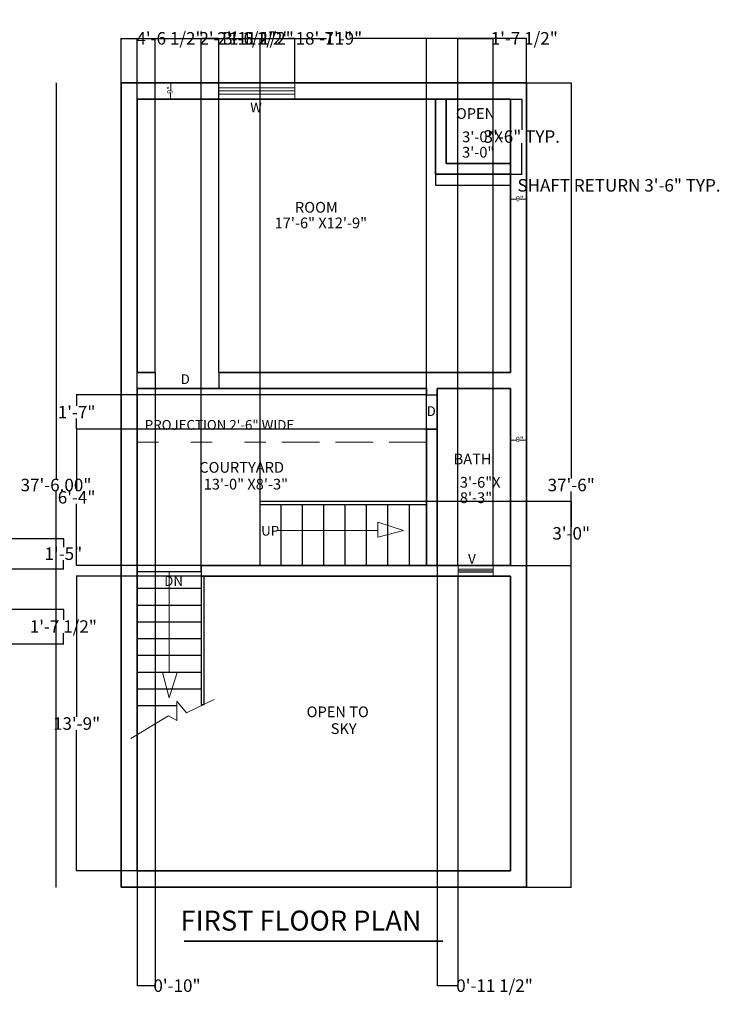
# Model space of a CAD drawing. Units: inches. Extents: x 193743 to 194406, y 400309 to 400860.
# Tile 2 of 2: x 194014 to 194406, y 400309 to 400860. Entities that reach past the tile are written whole.
import ezdxf

# ---------------------------------------------------------------- set-up
doc = ezdxf.new("R2010")
doc.units = ezdxf.units.IN
doc.header["$MEASUREMENT"] = 0
doc.linetypes.add('ACAD_ISO03W100', pattern=[30, 12, -18])
for name, color, linetype, lineweight in [('A-ANNO-DIMS', 2, 'Continuous', 18), ('A-ANNO-SYMB', 7, 'Continuous', 18), ('A-ANNO-TEXT', 7, 'Continuous', 18), ('A-ANNO-TITL', 7, 'Continuous', 35), ('A-AREA-IDEN', 7, 'Continuous', 18), ('A-DOOR', 3, 'Continuous', 25), ('A-FLOR-OVHD', 8, 'ACAD_ISO03W100', 18), ('A-FLOR-STRS', 7, 'Continuous', 25), ('A-GLAZ', 4, 'Continuous', 18), ('A-WALL', 7, 'Continuous', 35)]:
    doc.layers.add(name, color=color, linetype=linetype, lineweight=lineweight)
doc.styles.get("Standard").update_dxf_attribs({"font": 'arial.ttf'})
doc.dimstyles.get("Standard").update_dxf_attribs({"dimtxt": 7, "dimasz": 0.18, "dimexe": 0.18, "dimexo": 0.0625, "dimgap": 0.09, "dimtad": 0, "dimtih": 1, "dimtoh": 1, "dimzin": 0, "dimdsep": 46, "dimlunit": 3, "dimtxsty": 'Standard', "dimcen": 0.09, "dimadec": 0, "dimazin": 0, "dimtfac": 1, "dimtofl": 0, "dimtmove": 0, "dimatfit": 3, "dimfxl": 1, "dimtolj": 1, "dimtzin": 0, "dimarcsym": 0})

# ---------------------------------------------------------------- blocks, each defined once
blk = doc.blocks.new('*D2')
at = {"layer": 'A-ANNO-DIMS', "color": 0, "lineweight": -2, "transparency": 16777216}
for p, q in [((194034.37, 400824.24), (194034.71, 400824.24)), ((194034.53, 400824.06), (194034.53, 400602.91)), ((194034.53, 400374.42), (194034.53, 400595.57)), ((194034.37, 400374.24), (194034.71, 400374.24))]:
    blk.add_line(p, q, dxfattribs=at)
at = {"layer": 'A-ANNO-DIMS', "color": 0, "lineweight": 100, "transparency": 16777216}
for points in [[(194034.5, 400824.06), (194034.56, 400824.06), (194034.53, 400824.24)], [(194034.5, 400374.42), (194034.56, 400374.42), (194034.53, 400374.24)]]:
    blk.add_solid(points, dxfattribs=at)
at = {"layer": 'Defpoints', "color": 0, "lineweight": 100, "transparency": 16777216}
for p in [(194034.3, 400824.24), (194034.3, 400374.24), (194034.53, 400374.24)]:
    blk.add_point(p, dxfattribs=at)
at = {"layer": 'A-ANNO-DIMS', "color": 0, "transparency": 16777216, "insert": (194034.53, 400599.24), "char_height": 7, "attachment_point": 5}
blk.add_mtext('\\A1;37\'-6.00"', dxfattribs=at)
blk = doc.blocks.new('SHAFT-RETURN-36X36')
for p, q in [((0, 42), (0, 0)), ((6, 42), (6, 6)), ((6, 6), (42, 6)), ((0, 0), (42, 0))]:
    blk.add_line(p, q)
blk = doc.blocks.new('STAIR-DIRECTION-ARROW')
for p, q in [((3.8, 70.54), (3.8, 14.31)), ((0, 14.31), (8.31, 14.31)), ((3.8, 0), (0, 14.31)), ((8.31, 14.31), (3.8, 0))]:
    blk.add_line(p, q)
blk = doc.blocks.new('THICKNESS-9-H')
for p, q in [((0, 1.15), (3.54, 1.15)), ((5.14, 1.15), (9, 1.15))]:
    blk.add_line(p, q)
blk.add_text('9"', height=3).set_placement((2.97, 0))
blk = doc.blocks.new('THICKNESS-9-V')
for p, q in [((0.06, 9), (0.06, 5.01)), ((0, 3.6), (0, 0))]:
    blk.add_line(p, q)
blk.add_text('9"', height=3, rotation=90).set_placement((1.05, 2.9))
blk = doc.blocks.new('ROOM-TAG-OPEN-3X3')
for s, p in [('OPEN', (0, 21.67)), ('3\'-0"X', (3.49, 8.63)), ('3\'-0"', (3.46, 0))]:
    blk.add_text(s, height=6).set_placement(p)
blk = doc.blocks.new('*D10')
at = {"layer": 'A-ANNO-DIMS', "color": 0, "lineweight": -2, "transparency": 16777216}
for p, q in [((194247, 400773.18), (194247, 400766.76)), ((194289, 400773.18), (194289, 400766.76)), ((194247.18, 400766.94), (194288.82, 400766.94)), ((194289, 400766.94), (194289.18, 400766.94))]:
    blk.add_line(p, q, dxfattribs=at)
at = {"layer": 'A-ANNO-DIMS', "color": 0, "lineweight": 100, "transparency": 16777216}
for points in [[(194247.18, 400766.97), (194247.18, 400766.91), (194247, 400766.94)], [(194288.82, 400766.97), (194288.82, 400766.91), (194289, 400766.94)]]:
    blk.add_solid(points, dxfattribs=at)
at = {"layer": 'Defpoints', "color": 0, "lineweight": 100, "transparency": 16777216}
for p in [(194247, 400773.24), (194289, 400773.24), (194289, 400766.94)]:
    blk.add_point(p, dxfattribs=at)
at = {"layer": 'A-ANNO-DIMS', "color": 0, "transparency": 16777216, "insert": (194349.71, 400766.94), "char_height": 7, "attachment_point": 5}
blk.add_mtext('\\A1;SHAFT RETURN 3\'-6" TYP.', dxfattribs=at)
blk = doc.blocks.new('*D11')
at = {"layer": 'A-ANNO-DIMS', "color": 0, "lineweight": -2, "transparency": 16777216}
for p, q in [((194289.06, 400815.24), (194295.48, 400815.24)), ((194295.3, 400815.06), (194295.3, 400797.91)), ((194295.3, 400773.42), (194295.3, 400790.57)), ((194289.06, 400773.24), (194295.48, 400773.24))]:
    blk.add_line(p, q, dxfattribs=at)
at = {"layer": 'A-ANNO-DIMS', "color": 0, "lineweight": 100, "transparency": 16777216}
for points in [[(194295.27, 400815.06), (194295.33, 400815.06), (194295.3, 400815.24)], [(194295.27, 400773.42), (194295.33, 400773.42), (194295.3, 400773.24)]]:
    blk.add_solid(points, dxfattribs=at)
at = {"layer": 'Defpoints', "color": 0, "lineweight": 100, "transparency": 16777216}
for p in [(194289, 400815.24), (194295.3, 400815.24), (194289, 400773.24)]:
    blk.add_point(p, dxfattribs=at)
at = {"layer": 'A-ANNO-DIMS', "color": 0, "transparency": 16777216, "insert": (194295.3, 400794.24), "char_height": 7, "attachment_point": 5}
blk.add_mtext('\\A1;3\'-6" TYP.', dxfattribs=at)
blk = doc.blocks.new('*D14')
at = {"layer": 'A-ANNO-DIMS', "color": 0, "lineweight": -2, "transparency": 16777216}
for p, q in [((194071, 400824.3), (194071, 400849.37)), ((194071.18, 400849.19), (194170, 400849.19)), ((194297.82, 400849.19), (194199, 400849.19)), ((194298, 400824.3), (194298, 400849.37))]:
    blk.add_line(p, q, dxfattribs=at)
at = {"layer": 'A-ANNO-DIMS', "color": 0, "lineweight": 100, "transparency": 16777216}
for points in [[(194071.18, 400849.22), (194071.18, 400849.16), (194071, 400849.19)], [(194297.82, 400849.22), (194297.82, 400849.16), (194298, 400849.19)]]:
    blk.add_solid(points, dxfattribs=at)
at = {"layer": 'Defpoints', "color": 0, "lineweight": 100, "transparency": 16777216}
for p in [(194298, 400849.19), (194071, 400824.24), (194298, 400824.24)]:
    blk.add_point(p, dxfattribs=at)
at = {"layer": 'A-ANNO-DIMS', "color": 0, "transparency": 16777216, "insert": (194184.5, 400849.19), "char_height": 7, "attachment_point": 5}
blk.add_mtext('\\A1;18\'-11"', dxfattribs=at)
blk = doc.blocks.new('*D15')
at = {"layer": 'A-ANNO-DIMS', "color": 0, "lineweight": -2, "transparency": 16777216}
for p, q in [((194298.06, 400824.24), (194323.13, 400824.24)), ((194322.95, 400824.06), (194322.95, 400602.91)), ((194322.95, 400374.42), (194322.95, 400595.57)), ((194298.06, 400374.24), (194323.13, 400374.24))]:
    blk.add_line(p, q, dxfattribs=at)
at = {"layer": 'A-ANNO-DIMS', "color": 0, "lineweight": 100, "transparency": 16777216}
for points in [[(194322.92, 400824.06), (194322.98, 400824.06), (194322.95, 400824.24)], [(194322.92, 400374.42), (194322.98, 400374.42), (194322.95, 400374.24)]]:
    blk.add_solid(points, dxfattribs=at)
at = {"layer": 'Defpoints', "color": 0, "lineweight": 100, "transparency": 16777216}
for p in [(194298, 400824.24), (194322.95, 400824.24), (194298, 400374.24)]:
    blk.add_point(p, dxfattribs=at)
at = {"layer": 'A-ANNO-DIMS', "color": 0, "transparency": 16777216, "insert": (194322.95, 400599.24), "char_height": 7, "attachment_point": 5}
blk.add_mtext('\\A1;37\'-6"', dxfattribs=at)
blk = doc.blocks.new('*D16')
at = {"layer": 'A-ANNO-DIMS', "color": 0, "lineweight": -2, "transparency": 16777216}
for p, q in [((194071, 400824.3), (194071, 400849.37)), ((194071.18, 400849.19), (194080.67, 400849.19)), ((194125.54, 400849.19), (194116.05, 400849.19)), ((194125.72, 400824.3), (194125.72, 400849.37))]:
    blk.add_line(p, q, dxfattribs=at)
at = {"layer": 'A-ANNO-DIMS', "color": 0, "lineweight": 100, "transparency": 16777216}
for points in [[(194071.18, 400849.22), (194071.18, 400849.16), (194071, 400849.19)], [(194125.54, 400849.22), (194125.54, 400849.16), (194125.72, 400849.19)]]:
    blk.add_solid(points, dxfattribs=at)
at = {"layer": 'Defpoints', "color": 0, "lineweight": 100, "transparency": 16777216}
for p in [(194125.72, 400849.19), (194071, 400824.24), (194125.72, 400824.24)]:
    blk.add_point(p, dxfattribs=at)
at = {"layer": 'A-ANNO-DIMS', "color": 0, "transparency": 16777216, "insert": (194098.36, 400849.19), "char_height": 7, "attachment_point": 5}
blk.add_mtext('\\A1;4\'-6 1/2"', dxfattribs=at)
blk = doc.blocks.new('*D17')
at = {"layer": 'A-ANNO-DIMS', "color": 0, "lineweight": -2, "transparency": 16777216}
for p, q in [((194125.72, 400824.3), (194125.72, 400849.37)), ((194125.9, 400849.19), (194129.44, 400849.19)), ((194168.07, 400849.19), (194164.53, 400849.19)), ((194168.25, 400824.3), (194168.25, 400849.37))]:
    blk.add_line(p, q, dxfattribs=at)
at = {"layer": 'A-ANNO-DIMS', "color": 0, "lineweight": 100, "transparency": 16777216}
for points in [[(194125.9, 400849.22), (194125.9, 400849.16), (194125.72, 400849.19)], [(194168.07, 400849.22), (194168.07, 400849.16), (194168.25, 400849.19)]]:
    blk.add_solid(points, dxfattribs=at)
at = {"layer": 'Defpoints', "color": 0, "lineweight": 100, "transparency": 16777216}
for p in [(194168.25, 400849.19), (194125.72, 400824.24), (194168.25, 400824.24)]:
    blk.add_point(p, dxfattribs=at)
at = {"layer": 'A-ANNO-DIMS', "color": 0, "transparency": 16777216, "insert": (194146.98, 400849.19), "char_height": 7, "attachment_point": 5}
blk.add_mtext('\\A1;3\'-6 1/2"', dxfattribs=at)
blk = doc.blocks.new('*D28')
at = {"layer": 'A-ANNO-DIMS', "color": 0, "lineweight": -2, "transparency": 16777216}
for p, q in [((193849.76, 400569.32), (194038.83, 400569.32)), ((194038.65, 400569.14), (194038.65, 400564.44)), ((194038.65, 400552.42), (194038.65, 400557.12)), ((193849.76, 400552.24), (194038.83, 400552.24))]:
    blk.add_line(p, q, dxfattribs=at)
at = {"layer": 'A-ANNO-DIMS', "color": 0, "lineweight": 100, "transparency": 16777216}
for points in [[(194038.62, 400569.14), (194038.68, 400569.14), (194038.65, 400569.32)], [(194038.62, 400552.42), (194038.68, 400552.42), (194038.65, 400552.24)]]:
    blk.add_solid(points, dxfattribs=at)
at = {"layer": 'Defpoints', "color": 0, "lineweight": 100, "transparency": 16777216}
for p in [(193849.7, 400569.32), (194038.65, 400569.32), (193849.7, 400552.24)]:
    blk.add_point(p, dxfattribs=at)
at = {"layer": 'A-ANNO-DIMS', "color": 0, "transparency": 16777216, "insert": (194038.65, 400560.78), "char_height": 7, "attachment_point": 5}
blk.add_mtext('\\A1;1\'-5"', dxfattribs=at)
blk = doc.blocks.new('*D31')
at = {"layer": 'A-ANNO-DIMS', "color": 0, "lineweight": -2, "transparency": 16777216}
for p, q in [((193849.76, 400529.76), (194038.83, 400529.76)), ((194038.65, 400529.58), (194038.65, 400523.75)), ((194038.65, 400510.5), (194038.65, 400516.33)), ((193849.76, 400510.32), (194038.83, 400510.32))]:
    blk.add_line(p, q, dxfattribs=at)
at = {"layer": 'A-ANNO-DIMS', "color": 0, "lineweight": 100, "transparency": 16777216}
for points in [[(194038.62, 400529.58), (194038.68, 400529.58), (194038.65, 400529.76)], [(194038.62, 400510.5), (194038.68, 400510.5), (194038.65, 400510.32)]]:
    blk.add_solid(points, dxfattribs=at)
at = {"layer": 'Defpoints', "color": 0, "lineweight": 100, "transparency": 16777216}
for p in [(193849.7, 400529.76), (193849.7, 400510.32), (194038.65, 400510.32)]:
    blk.add_point(p, dxfattribs=at)
at = {"layer": 'A-ANNO-DIMS', "color": 0, "transparency": 16777216, "insert": (194038.65, 400520.04), "char_height": 7, "attachment_point": 5}
blk.add_mtext('\\A1;1\'-7 1/2"', dxfattribs=at)
blk = doc.blocks.new('*D36')
at = {"layer": 'A-ANNO-DIMS', "color": 0, "lineweight": -2, "transparency": 16777216}
for p, q in [((194080, 400653.18), (194080, 400318.88)), ((194089.98, 400653.18), (194089.98, 400318.88)), ((194080.18, 400319.06), (194089.8, 400319.06)), ((194089.98, 400319.06), (194090.16, 400319.06))]:
    blk.add_line(p, q, dxfattribs=at)
at = {"layer": 'A-ANNO-DIMS', "color": 0, "lineweight": 100, "transparency": 16777216}
for points in [[(194080.18, 400319.09), (194080.18, 400319.03), (194080, 400319.06)], [(194089.8, 400319.09), (194089.8, 400319.03), (194089.98, 400319.06)]]:
    blk.add_solid(points, dxfattribs=at)
at = {"layer": 'Defpoints', "color": 0, "lineweight": 100, "transparency": 16777216}
for p in [(194080, 400653.24), (194089.98, 400653.24), (194089.98, 400319.06)]:
    blk.add_point(p, dxfattribs=at)
at = {"layer": 'A-ANNO-DIMS', "color": 0, "transparency": 16777216, "insert": (194102.27, 400319.06), "char_height": 7, "attachment_point": 5}
blk.add_mtext('\\A1;0\'-10"', dxfattribs=at)
blk = doc.blocks.new('*D37')
at = {"layer": 'A-ANNO-DIMS', "color": 0, "lineweight": -2, "transparency": 16777216}
for p, q in [((194089.98, 400662.3), (194089.98, 400849.37)), ((194090.16, 400849.19), (194125.53, 400849.19)), ((194125.71, 400662.3), (194125.71, 400849.37)), ((194125.71, 400849.19), (194125.89, 400849.19))]:
    blk.add_line(p, q, dxfattribs=at)
at = {"layer": 'A-ANNO-DIMS', "color": 0, "lineweight": 100, "transparency": 16777216}
for points in [[(194090.16, 400849.22), (194090.16, 400849.16), (194089.98, 400849.19)], [(194125.53, 400849.22), (194125.53, 400849.16), (194125.71, 400849.19)]]:
    blk.add_solid(points, dxfattribs=at)
at = {"layer": 'Defpoints', "color": 0, "lineweight": 100, "transparency": 16777216}
for p in [(194125.71, 400849.19), (194089.98, 400662.24), (194125.71, 400662.24)]:
    blk.add_point(p, dxfattribs=at)
at = {"layer": 'A-ANNO-DIMS', "color": 0, "transparency": 16777216, "insert": (194146.22, 400849.19), "char_height": 7, "attachment_point": 5}
blk.add_mtext('\\A1;2\'-11 1/2"', dxfattribs=at)
blk = doc.blocks.new('*D38')
at = {"layer": 'A-ANNO-DIMS', "color": 0, "lineweight": -2, "transparency": 16777216}
for p, q in [((194241.94, 400649.64), (194045.87, 400649.64)), ((194046.05, 400649.46), (194046.05, 400643.63)), ((194046.05, 400630.59), (194046.05, 400636.42)), ((194241.94, 400630.41), (194045.87, 400630.41))]:
    blk.add_line(p, q, dxfattribs=at)
at = {"layer": 'A-ANNO-DIMS', "color": 0, "lineweight": 100, "transparency": 16777216}
for points in [[(194046.02, 400649.46), (194046.08, 400649.46), (194046.05, 400649.64)], [(194046.02, 400630.59), (194046.08, 400630.59), (194046.05, 400630.41)]]:
    blk.add_solid(points, dxfattribs=at)
at = {"layer": 'Defpoints', "color": 0, "lineweight": 100, "transparency": 16777216}
for p in [(194046.05, 400649.64), (194242, 400649.64), (194242, 400630.41)]:
    blk.add_point(p, dxfattribs=at)
at = {"layer": 'A-ANNO-DIMS', "color": 0, "transparency": 16777216, "insert": (194046.05, 400640.02), "char_height": 7, "attachment_point": 5}
blk.add_mtext('\\A1;1\'-7"', dxfattribs=at)
blk = doc.blocks.new('*D39')
at = {"layer": 'A-ANNO-DIMS', "color": 0, "lineweight": -2, "transparency": 16777216}
for p, q in [((194247.94, 400630.41), (194045.87, 400630.41)), ((194046.05, 400630.23), (194046.05, 400595.99)), ((194046.05, 400554.42), (194046.05, 400588.66)), ((194247.94, 400554.24), (194045.87, 400554.24))]:
    blk.add_line(p, q, dxfattribs=at)
at = {"layer": 'A-ANNO-DIMS', "color": 0, "lineweight": 100, "transparency": 16777216}
for points in [[(194046.02, 400630.23), (194046.08, 400630.23), (194046.05, 400630.41)], [(194046.02, 400554.42), (194046.08, 400554.42), (194046.05, 400554.24)]]:
    blk.add_solid(points, dxfattribs=at)
at = {"layer": 'Defpoints', "color": 0, "lineweight": 100, "transparency": 16777216}
for p in [(194046.05, 400630.41), (194248, 400630.41), (194248, 400554.24)]:
    blk.add_point(p, dxfattribs=at)
at = {"layer": 'A-ANNO-DIMS', "color": 0, "transparency": 16777216, "insert": (194046.05, 400592.33), "char_height": 7, "attachment_point": 5}
blk.add_mtext('\\A1;6\'-4"', dxfattribs=at)
blk = doc.blocks.new('*D40')
at = {"layer": 'A-ANNO-DIMS', "color": 0, "lineweight": -2, "transparency": 16777216}
for p, q in [((194259.57, 400554.3), (194259.57, 400849.37)), ((194259.75, 400849.19), (194279.09, 400849.19)), ((194279.27, 400554.3), (194279.27, 400849.37)), ((194279.27, 400849.19), (194279.45, 400849.19))]:
    blk.add_line(p, q, dxfattribs=at)
at = {"layer": 'A-ANNO-DIMS', "color": 0, "lineweight": 100, "transparency": 16777216}
for points in [[(194259.75, 400849.22), (194259.75, 400849.16), (194259.57, 400849.19)], [(194279.09, 400849.22), (194279.09, 400849.16), (194279.27, 400849.19)]]:
    blk.add_solid(points, dxfattribs=at)
at = {"layer": 'Defpoints', "color": 0, "lineweight": 100, "transparency": 16777216}
for p in [(194279.27, 400849.19), (194259.57, 400554.24), (194279.27, 400554.24)]:
    blk.add_point(p, dxfattribs=at)
at = {"layer": 'A-ANNO-DIMS', "color": 0, "transparency": 16777216, "insert": (194296.67, 400849.19), "char_height": 7, "attachment_point": 5}
blk.add_mtext('\\A1;1\'-7 1/2"', dxfattribs=at)
blk = doc.blocks.new('*D41')
at = {"layer": 'A-ANNO-DIMS', "color": 0, "lineweight": -2, "transparency": 16777216}
for p, q in [((194248, 400554.18), (194248, 400318.88)), ((194259.57, 400548.18), (194259.57, 400318.88)), ((194248.18, 400319.06), (194259.39, 400319.06)), ((194259.57, 400319.06), (194259.75, 400319.06))]:
    blk.add_line(p, q, dxfattribs=at)
at = {"layer": 'A-ANNO-DIMS', "color": 0, "lineweight": 100, "transparency": 16777216}
for points in [[(194248.18, 400319.09), (194248.18, 400319.03), (194248, 400319.06)], [(194259.39, 400319.09), (194259.39, 400319.03), (194259.57, 400319.06)]]:
    blk.add_solid(points, dxfattribs=at)
at = {"layer": 'Defpoints', "color": 0, "lineweight": 100, "transparency": 16777216}
for p in [(194248, 400554.24), (194259.57, 400548.24), (194259.57, 400319.06)]:
    blk.add_point(p, dxfattribs=at)
at = {"layer": 'A-ANNO-DIMS', "color": 0, "transparency": 16777216, "insert": (194280.02, 400319.06), "char_height": 7, "attachment_point": 5}
blk.add_mtext('\\A1;0\'-11 1/2"', dxfattribs=at)
blk = doc.blocks.new('*D42')
at = {"layer": 'A-ANNO-DIMS', "color": 0, "lineweight": -2, "transparency": 16777216}
for p, q in [((194148.76, 400590.18), (194148.76, 400849.37)), ((194148.94, 400849.19), (194186.02, 400849.19)), ((194241.82, 400849.19), (194204.75, 400849.19)), ((194242, 400590.18), (194242, 400849.37))]:
    blk.add_line(p, q, dxfattribs=at)
at = {"layer": 'A-ANNO-DIMS', "color": 0, "lineweight": 100, "transparency": 16777216}
for points in [[(194148.94, 400849.22), (194148.94, 400849.16), (194148.76, 400849.19)], [(194241.82, 400849.22), (194241.82, 400849.16), (194242, 400849.19)]]:
    blk.add_solid(points, dxfattribs=at)
at = {"layer": 'Defpoints', "color": 0, "lineweight": 100, "transparency": 16777216}
for p in [(194242, 400849.19), (194148.76, 400590.12), (194242, 400590.12)]:
    blk.add_point(p, dxfattribs=at)
at = {"layer": 'A-ANNO-DIMS', "color": 0, "transparency": 16777216, "insert": (194195.38, 400849.19), "char_height": 7, "attachment_point": 5}
blk.add_mtext('\\A1;7\'-9"', dxfattribs=at)
blk = doc.blocks.new('*D43')
at = {"layer": 'A-ANNO-DIMS', "color": 0, "lineweight": -2, "transparency": 16777216}
for p, q in [((194242.06, 400590.12), (194323.13, 400590.12)), ((194322.95, 400589.94), (194322.95, 400575.85)), ((194322.95, 400554.42), (194322.95, 400568.51)), ((194242.06, 400554.24), (194323.13, 400554.24))]:
    blk.add_line(p, q, dxfattribs=at)
at = {"layer": 'A-ANNO-DIMS', "color": 0, "lineweight": 100, "transparency": 16777216}
for points in [[(194322.92, 400589.94), (194322.98, 400589.94), (194322.95, 400590.12)], [(194322.92, 400554.42), (194322.98, 400554.42), (194322.95, 400554.24)]]:
    blk.add_solid(points, dxfattribs=at)
at = {"layer": 'Defpoints', "color": 0, "lineweight": 100, "transparency": 16777216}
for p in [(194242, 400590.12), (194322.95, 400590.12), (194242, 400554.24)]:
    blk.add_point(p, dxfattribs=at)
at = {"layer": 'A-ANNO-DIMS', "color": 0, "transparency": 16777216, "insert": (194322.95, 400572.18), "char_height": 7, "attachment_point": 5}
blk.add_mtext('\\A1;3\'-0"', dxfattribs=at)
blk = doc.blocks.new('*D44')
at = {"layer": 'A-ANNO-DIMS', "color": 0, "lineweight": -2, "transparency": 16777216}
for p, q in [((194080, 400550.66), (194080, 400849.37)), ((194080.18, 400849.19), (194115.57, 400849.19)), ((194115.75, 400550.66), (194115.75, 400849.37)), ((194115.75, 400849.19), (194115.93, 400849.19))]:
    blk.add_line(p, q, dxfattribs=at)
at = {"layer": 'A-ANNO-DIMS', "color": 0, "lineweight": 100, "transparency": 16777216}
for points in [[(194080.18, 400849.22), (194080.18, 400849.16), (194080, 400849.19)], [(194115.57, 400849.22), (194115.57, 400849.16), (194115.75, 400849.19)]]:
    blk.add_solid(points, dxfattribs=at)
at = {"layer": 'Defpoints', "color": 0, "lineweight": 100, "transparency": 16777216}
for p in [(194115.75, 400849.19), (194080, 400550.6), (194115.75, 400550.6)]:
    blk.add_point(p, dxfattribs=at)
at = {"layer": 'A-ANNO-DIMS', "color": 0, "transparency": 16777216, "insert": (194136.26, 400849.19), "char_height": 7, "attachment_point": 5}
blk.add_mtext('\\A1;2\'-11 1/2"', dxfattribs=at)
blk = doc.blocks.new('*D45')
at = {"layer": 'A-ANNO-DIMS', "color": 0, "lineweight": -2, "transparency": 16777216}
for p, q in [((194115.69, 400548.24), (194045.87, 400548.24)), ((194046.05, 400548.06), (194046.05, 400469.41)), ((194046.05, 400383.42), (194046.05, 400462.07)), ((194079.94, 400383.24), (194045.87, 400383.24))]:
    blk.add_line(p, q, dxfattribs=at)
at = {"layer": 'A-ANNO-DIMS', "color": 0, "lineweight": 100, "transparency": 16777216}
for points in [[(194046.02, 400548.06), (194046.08, 400548.06), (194046.05, 400548.24)], [(194046.02, 400383.42), (194046.08, 400383.42), (194046.05, 400383.24)]]:
    blk.add_solid(points, dxfattribs=at)
at = {"layer": 'Defpoints', "color": 0, "lineweight": 100, "transparency": 16777216}
for p in [(194046.05, 400548.24), (194115.75, 400548.24), (194080, 400383.24)]:
    blk.add_point(p, dxfattribs=at)
at = {"layer": 'A-ANNO-DIMS', "color": 0, "transparency": 16777216, "insert": (194046.05, 400465.74), "char_height": 7, "attachment_point": 5}
blk.add_mtext('\\A1;13\'-9"', dxfattribs=at)

msp = doc.modelspace()

# ---------------------------------------------------------------- linework, layer by layer
at = {"layer": 'A-ANNO-SYMB'}
for p, q in [((194102.168, 400467.422), (194102.168, 400478.247)), ((194102.168, 400478.247), (194107.51, 400471.707)), ((194107.51, 400471.707), (194123.162, 400479.225)), ((194076.35, 400457.378), (194097.483, 400470.045)), ((194097.483, 400470.045), (194102.168, 400467.422))]:
    msp.add_line(p, q, dxfattribs=at)
at = {"layer": 'A-ANNO-TITL'}
msp.add_line((194106.356, 400344.014), (194251.085, 400344.014), dxfattribs=at)
at = {"layer": 'A-DOOR'}
for p, q in [((194089.979, 400662.24), (194089.979, 400653.24)), ((194125.711, 400662.24), (194125.711, 400653.24)), ((194242.002, 400649.635), (194248.002, 400649.635)), ((194242.002, 400630.41), (194248.002, 400630.41))]:
    msp.add_line(p, q, dxfattribs=at)
at = {"layer": 'A-FLOR-OVHD'}
for p, q in [((194242.002, 400623.24), (194080.002, 400623.24)), ((194161.002, 400623.24), (194242.002, 400623.24))]:
    msp.add_line(p, q, dxfattribs=at)
at = {"layer": 'A-FLOR-STRS'}
for p, q in [((194148.765, 400588.401), (194148.765, 400590.121)), ((194148.765, 400590.121), (194242.002, 400590.121)), ((194148.765, 400554.24), (194148.765, 400588.401)), ((194148.765, 400588.401), (194242.002, 400588.401)), ((194160.314, 400588.401), (194160.314, 400554.24)), ((194172.291, 400588.401), (194172.291, 400554.24)), ((194184.267, 400588.401), (194184.267, 400554.24)), ((194196.244, 400588.401), (194196.244, 400554.24)), ((194208.22, 400588.401), (194208.22, 400554.24)), ((194220.197, 400588.401), (194220.197, 400554.24)), ((194232.173, 400588.401), (194232.173, 400554.24)), ((194115.751, 400554.24), (194115.751, 400476.489)), ((194115.751, 400550.6), (194080.002, 400550.6)), ((194117.468, 400476.489), (194117.468, 400548.24)), ((194115.751, 400541.229), (194080.002, 400541.229)), ((194115.751, 400531.859), (194080.002, 400531.859)), ((194115.751, 400522.488), (194080.002, 400522.488)), ((194115.751, 400513.118), (194080.002, 400513.118)), ((194115.751, 400503.748), (194080.002, 400503.748)), ((194115.751, 400494.377), (194080.002, 400494.377)), ((194115.751, 400485.007), (194080.002, 400485.007)), ((194102.168, 400475.637), (194080.002, 400475.637)), ((194115.751, 400475.637), (194115.691, 400475.637)), ((194115.751, 400476.489), (194117.468, 400476.489))]:
    msp.add_line(p, q, dxfattribs=at)
at = {"layer": 'A-GLAZ'}
for p, q in [((194125.715, 400824.24), (194125.715, 400815.24)), ((194125.715, 400821.556), (194168.249, 400821.556)), ((194168.249, 400824.24), (194168.249, 400815.24)), ((194125.715, 400819.74), (194168.249, 400819.74)), ((194125.715, 400817.968), (194168.249, 400817.968)), ((194259.575, 400554.24), (194259.575, 400548.24)), ((194279.267, 400554.24), (194259.575, 400554.24)), ((194259.575, 400554.24), (194259.575, 400552.106)), ((194259.575, 400552.106), (194279.267, 400552.106)), ((194279.267, 400548.24), (194279.267, 400554.24)), ((194279.267, 400552.106), (194279.267, 400551.24)), ((194279.267, 400551.24), (194259.575, 400551.24)), ((194259.575, 400551.24), (194259.575, 400550.376)), ((194259.575, 400550.376), (194279.267, 400550.376)), ((194259.575, 400548.24), (194279.267, 400548.24))]:
    msp.add_line(p, q, dxfattribs=at)
at = {"layer": 'A-WALL'}
for p, q in [((194071.002, 400824.24), (194298.002, 400824.24)), ((194071.002, 400374.24), (194071.002, 400824.24)), ((194298.002, 400824.24), (194298.002, 400374.24)), ((194080.002, 400815.24), (194289.002, 400815.24)), ((194080.002, 400662.24), (194080.002, 400815.24)), ((194289.002, 400815.24), (194289.002, 400662.24)), ((194080.002, 400662.24), (194089.979, 400662.24)), ((194125.711, 400662.24), (194289.002, 400662.24)), ((194080.002, 400383.24), (194080.002, 400653.24)), ((194080.002, 400653.24), (194242.002, 400653.24)), ((194242.002, 400653.24), (194242.002, 400649.635)), ((194248.002, 400554.24), (194248.002, 400653.24)), ((194248.002, 400653.24), (194289.002, 400653.24)), ((194289.002, 400653.24), (194289.002, 400554.24)), ((194242.002, 400554.24), (194242.002, 400630.41)), ((194115.751, 400554.24), (194242.002, 400554.24)), ((194248.002, 400554.24), (194289.002, 400554.24)), ((194115.751, 400548.24), (194289.002, 400548.24)), ((194289.002, 400548.24), (194289.002, 400383.24)), ((194289.002, 400383.24), (194080.002, 400383.24)), ((194298.002, 400374.24), (194071.002, 400374.24))]:
    msp.add_line(p, q, dxfattribs=at)

# ---------------------------------------------------------------- block references
at = {"layer": 'A-ANNO-DIMS'}
for name, p in [('THICKNESS-9-V', (194098.685, 400815.24)), ('THICKNESS-9-H', (194289.002, 400757.997)), ('THICKNESS-9-H', (194289.002, 400623.235))]:
    msp.add_blockref(name, p, dxfattribs=at)
at = {"layer": 'A-ANNO-SYMB', "rotation": 89.99999999990492}
msp.add_blockref('STAIR-DIRECTION-ARROW', (194229.043, 400570.058), dxfattribs=at)
at = {"layer": 'A-ANNO-SYMB'}
msp.add_blockref('STAIR-DIRECTION-ARROW', (194094.079, 400480.063), dxfattribs=at)
at = {"layer": 'A-AREA-IDEN'}
msp.add_blockref('ROOM-TAG-OPEN-3X3', (194258.404, 400782.458), dxfattribs=at)
at = {"layer": 'A-WALL'}
msp.add_blockref('SHAFT-RETURN-36X36', (194247.002, 400773.24), dxfattribs=at)

# ---------------------------------------------------------------- texts
at = {"layer": 'A-ANNO-TEXT'}
for s, height, p in [('W', 5.457, (194143.263, 400807.813)), ('D', 5.457, (194104.32, 400655.738)), ('D', 5.457, (194242.002, 400637.833)), ('PROJECTION 2\'-6" WIDE', 5.45728, (194084.247, 400630.15)), ('UP', 5.4573, (194149.393, 400570.916)), ('V', 5.457, (194265.233, 400555.129)), ('DN', 5.4573, (194095.113, 400542.797))]:
    msp.add_text(s, height=height, dxfattribs=at).set_placement(p)
at = {"layer": 'A-ANNO-TITL'}
msp.add_text('FIRST FLOOR PLAN', height=11.181, dxfattribs=at).set_placement((194104.249, 400349.87))
at = {"layer": 'A-AREA-IDEN'}
for s, p in [('ROOM', (194168.302, 400751.636)), ('17\'-6" X12\'-9"', (194156.902, 400742.895)), ('COURTYARD', (194114.724, 400606.11)), ('BATH', (194257.138, 400610.793)), ('13\'-0" X8\'-3"', (194117.202, 400596.715)), ('3\'-6"X', (194260.624, 400597.753)), ('8\'-3"', (194260.604, 400589.12)), ('OPEN TO', (194174.841, 400469.296)), ('SKY', (194188.317, 400459.901))]:
    msp.add_text(s, height=6, dxfattribs=at).set_placement(p)

# ---------------------------------------------------------------- dimensions: what is measured, and where the dimension line sits
at = {"layer": 'A-ANNO-DIMS'}
for base, p1, p2, picture, middle in [((194125.715, 400849.19), (194071.002, 400824.24), (194125.715, 400824.24), '*D16', (194098.359, 400849.19)), ((194115.751, 400849.19), (194080.002, 400550.6), (194115.751, 400550.6), '*D44', (194136.26, 400849.19)), ((194125.711, 400849.19), (194089.979, 400662.24), (194125.711, 400662.24), '*D37', (194146.22, 400849.19)), ((194168.249, 400849.19), (194125.715, 400824.24), (194168.249, 400824.24), '*D17', (194146.982, 400849.19)), ((194279.267, 400849.19), (194259.575, 400554.24), (194279.267, 400554.24), '*D40', (194296.667, 400849.19)), ((194298.002, 400849.19), (194071.002, 400824.24), (194298.002, 400824.24), '*D14', (194184.502, 400849.19)), ((194242.002, 400849.19), (194148.765, 400590.121), (194242.002, 400590.121), '*D42', (194195.383, 400849.19)), ((194089.979, 400319.064), (194080.002, 400653.24), (194089.979, 400653.24), '*D36', (194102.272, 400319.064)), ((194259.575, 400319.064), (194248.002, 400554.24), (194259.575, 400548.24), '*D41', (194280.023, 400319.064))]:
    dim = msp.add_linear_dim(base=base, p1=p1, p2=p2, dimstyle='Standard', override={"dimdec": 1, "dimlfac": 1, "dimrnd": 0, "dimzin": 1, "dimdsep": 46, "dimlunit": 4, "dimfrac": 2}, dxfattribs=at)
    dim.commit()
    dim.dimension.update_dxf_attribs({"geometry": picture, "text_midpoint": middle})
for base, p1, p2, override, picture, middle in [((194034.528, 400374.24), (194034.304, 400824.24), (194034.304, 400374.24), {"dimclrd": 0, "dimclre": 0, "dimclrt": 0}, '*D2', (194034.528, 400599.24)), ((194322.952, 400824.24), (194298.002, 400374.24), (194298.002, 400824.24), {"dimdec": 1, "dimlfac": 1, "dimrnd": 0, "dimzin": 1, "dimdsep": 46, "dimlunit": 4, "dimfrac": 2}, '*D15', (194322.952, 400599.24)), ((194046.052, 400649.635), (194242.002, 400630.41), (194242.002, 400649.635), {"dimdec": 1, "dimlfac": 1, "dimrnd": 0, "dimzin": 1, "dimdsep": 46, "dimlunit": 4, "dimfrac": 2}, '*D38', (194046.052, 400640.023)), ((194046.052, 400630.41), (194248.002, 400554.24), (194248.002, 400630.41), {"dimdec": 1, "dimlfac": 1, "dimrnd": 0, "dimzin": 1, "dimdsep": 46, "dimlunit": 4, "dimfrac": 2}, '*D39', (194046.052, 400592.325)), ((194322.952, 400590.121), (194242.002, 400554.24), (194242.002, 400590.121), {"dimdec": 1, "dimlfac": 1, "dimrnd": 0, "dimzin": 1, "dimdsep": 46, "dimlunit": 4, "dimfrac": 2}, '*D43', (194322.952, 400572.18)), ((194038.647, 400569.318), (193849.697, 400552.24), (193849.697, 400569.318), {"dimdec": 1, "dimlfac": 1, "dimrnd": 0, "dimzin": 1, "dimdsep": 46, "dimlunit": 4, "dimfrac": 2}, '*D28', (194038.647, 400560.779)), ((194046.052, 400548.24), (194080.002, 400383.24), (194115.751, 400548.24), {"dimdec": 1, "dimlfac": 1, "dimrnd": 0, "dimzin": 1, "dimdsep": 46, "dimlunit": 4, "dimfrac": 2}, '*D45', (194046.052, 400465.74)), ((194038.647, 400510.321), (193849.697, 400529.763), (193849.697, 400510.321), {"dimdec": 1, "dimlfac": 1, "dimrnd": 0, "dimzin": 1, "dimdsep": 46, "dimlunit": 4, "dimfrac": 2}, '*D31', (194038.647, 400520.042))]:
    dim = msp.add_linear_dim(base=base, p1=p1, p2=p2, angle=90, dimstyle='Standard', override=override, dxfattribs=at)
    dim.commit()
    dim.dimension.update_dxf_attribs({"geometry": picture, "text_midpoint": middle})
dim = msp.add_linear_dim(base=(194295.302, 400815.24), p1=(194289.002, 400773.24), p2=(194289.002, 400815.24), angle=90, text='<> TYP.', dimstyle='Standard', override={"dimdec": 1, "dimlfac": 1, "dimrnd": 0, "dimzin": 1, "dimdsep": 46, "dimlunit": 4, "dimfrac": 2}, dxfattribs=at)
dim.commit()
dim.dimension.update_dxf_attribs({"geometry": '*D11', "text_midpoint": (194295.302, 400794.24)})
dim = msp.add_linear_dim(base=(194289.002, 400766.94), p1=(194247.002, 400773.24), p2=(194289.002, 400773.24), text='SHAFT RETURN <> TYP.', dimstyle='Standard', override={"dimdec": 1, "dimlfac": 1, "dimrnd": 0, "dimzin": 1, "dimdsep": 46, "dimlunit": 4, "dimfrac": 2}, dxfattribs=at)
dim.commit()
dim.dimension.update_dxf_attribs({"geometry": '*D10', "text_midpoint": (194349.705, 400766.94)})

doc.saveas('drawing.dxf')
